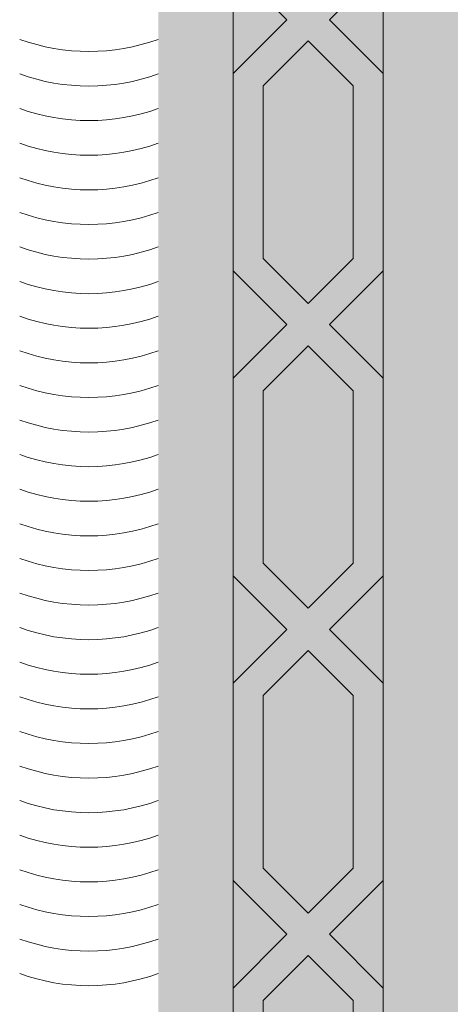
# Model space of a CAD drawing. Units: inches. Extents: x 844 to 2234, y 346 to 1084.
# Tile 27 of 93: x 1249.183 to 1252.862, y 687.38 to 695.763. Entities that reach past the tile are written whole.
import ezdxf

# ---------------------------------------------------------------- set-up
doc = ezdxf.new("R2010")
doc.units = ezdxf.units.IN
doc.header["$MEASUREMENT"] = 0
doc.layers.add('furniture', color=8, linetype='Continuous', lineweight=18)
doc.layers.add('RA-AP-01$0$INT', color=35, linetype='Continuous', lineweight=5)
doc.layers.add('RA-AP-01$0$FURN', color=3, linetype='Continuous')

# ---------------------------------------------------------------- blocks, each defined once
blk = doc.blocks.new('A$C18D01794')
at = {"layer": 'RA-AP-01$0$INT'}
h = blk.add_hatch(color=256, dxfattribs=at)
h.paths.add_polyline_path([(4.35521, -6.15671), (4.35521, -8.05671), (5.45521, -8.05671), (5.45521, -6.15671)])
h.paths.add_polyline_path([(4.40521, -8.00671), (4.40521, -6.20671), (5.40521, -6.20671), (5.40521, -8.00671)], flags=16)
h = blk.add_hatch(color=256, dxfattribs=at)
h.paths.add_polyline_path([(4.46935, -7.07085), (4.50521, -7.035), (4.50521, -7.10671)])
h.paths.add_polyline_path([(4.45521, -7.085), (4.47692, -7.10671), (4.43349, -7.10671)])
h.paths.add_polyline_path([(4.40521, -7.035), (4.44106, -7.07085), (4.40521, -7.10671)])
h.paths.add_polyline_path([(4.42521, -6.91146), (4.45521, -6.88146), (4.48521, -6.91146), (4.48521, -7.02671), (4.45521, -7.05671), (4.42521, -7.02671)])
h.paths.add_polyline_path([(4.50521, -6.83146), (4.50521, -6.90318), (4.46935, -6.86732)])
h.paths.add_polyline_path([(4.42521, -6.70793), (4.45521, -6.67793), (4.48521, -6.70793), (4.48521, -6.82318), (4.45521, -6.85318), (4.42521, -6.82318)])
h.paths.add_polyline_path([(4.42521, -6.50439), (4.45521, -6.47439), (4.48521, -6.50439), (4.48521, -6.61964), (4.45521, -6.64964), (4.42521, -6.61964)])
h.paths.add_polyline_path([(4.46935, -6.66378), (4.50521, -6.62793), (4.50521, -6.69964)])
h.paths.add_polyline_path([(4.40521, -6.62793), (4.44106, -6.66378), (4.40521, -6.69964)])
h.paths.add_polyline_path([(4.40521, -6.42439), (4.44106, -6.46025), (4.40521, -6.49611)])
h.paths.add_polyline_path([(4.46935, -6.46025), (4.50521, -6.42439), (4.50521, -6.49611)])
h.paths.add_polyline_path([(4.42521, -6.30085), (4.45521, -6.27085), (4.48521, -6.30085), (4.48521, -6.41611), (4.45521, -6.44611), (4.42521, -6.41611)])
h.paths.add_polyline_path([(4.42521, -6.22671), (4.47106, -6.22671), (4.42521, -6.27257)])
h.paths.add_polyline_path([(4.49935, -6.22671), (4.63606, -6.22671), (4.66606, -6.25671), (4.63606, -6.28671), (4.49935, -6.28671), (4.46935, -6.25671)])
h.paths.add_polyline_path([(4.68021, -6.27085), (4.71606, -6.30671), (4.64435, -6.30671)])
h.paths.add_polyline_path([(4.64435, -6.20671), (4.71606, -6.20671), (4.68021, -6.24257)])
h.paths.add_polyline_path([(4.72435, -6.22671), (4.86106, -6.22671), (4.89106, -6.25671), (4.86106, -6.28671), (4.72435, -6.28671), (4.69435, -6.25671)])
h.paths.add_polyline_path([(4.90521, -6.27085), (4.94106, -6.30671), (4.86935, -6.30671)])
h.paths.add_polyline_path([(4.86935, -6.20671), (4.94106, -6.20671), (4.90521, -6.24257)])
h.paths.add_polyline_path([(4.94935, -6.22671), (5.08606, -6.22671), (5.11606, -6.25671), (5.08606, -6.28671), (4.94935, -6.28671), (4.91935, -6.25671)])
h.paths.add_polyline_path([(5.13021, -6.27085), (5.16606, -6.30671), (5.09435, -6.30671)])
h.paths.add_polyline_path([(5.09435, -6.20671), (5.16606, -6.20671), (5.13021, -6.24257)])
h.paths.add_polyline_path([(5.17435, -6.22671), (5.31106, -6.22671), (5.34106, -6.25671), (5.31106, -6.28671), (5.17435, -6.28671), (5.14435, -6.25671)])
h.paths.add_polyline_path([(5.32521, -6.30085), (5.35521, -6.27085), (5.38521, -6.30085), (5.38521, -6.41611), (5.35521, -6.44611), (5.32521, -6.41611)])
h.paths.add_polyline_path([(5.33935, -6.22671), (5.38521, -6.22671), (5.38521, -6.27257)])
h.paths.add_polyline_path([(5.32521, -6.50439), (5.35521, -6.47439), (5.38521, -6.50439), (5.38521, -6.61964), (5.35521, -6.64964), (5.32521, -6.61964)])
h.paths.add_polyline_path([(5.30521, -6.42439), (5.34106, -6.46025), (5.30521, -6.49611)])
h.paths.add_polyline_path([(5.36935, -6.46025), (5.40521, -6.42439), (5.40521, -6.49611)])
h.paths.add_polyline_path([(5.40521, -6.62793), (5.40521, -6.69964), (5.36935, -6.66378)])
h.paths.add_polyline_path([(5.30521, -6.62793), (5.34106, -6.66378), (5.30521, -6.69964)])
h.paths.add_polyline_path([(5.32521, -6.70793), (5.35521, -6.67793), (5.38521, -6.70793), (5.38521, -6.82318), (5.35521, -6.85318), (5.32521, -6.82318)])
h.paths.add_polyline_path([(5.30521, -6.83146), (5.34106, -6.86732), (5.30521, -6.90318)])
h.paths.add_polyline_path([(5.32521, -6.91146), (5.35521, -6.88146), (5.38521, -6.91146), (5.38521, -7.02671), (5.35521, -7.05671), (5.32521, -7.02671)])
h.paths.add_polyline_path([(5.40458, -6.83209, 0.001218), (5.40521, -6.83231), (5.40521, -6.90318), (5.36935, -6.86732)])
h.paths.add_polyline_path([(5.36935, -7.07085), (5.40521, -7.035), (5.40521, -7.10671)])
h.paths.add_polyline_path([(5.35521, -7.085), (5.37692, -7.10671), (5.33349, -7.10671)])
h.paths.add_polyline_path([(5.30521, -7.035), (5.34106, -7.07085), (5.30521, -7.10671)])
h = blk.add_hatch(color=256, dxfattribs=at)
h.paths.add_polyline_path([(4.50521, -6.62793), (4.46935, -6.66378), (4.50521, -6.69964), (4.50521, -6.83146), (4.46935, -6.86732), (4.50521, -6.90318), (4.50521, -7.035), (4.46935, -7.07085), (4.50521, -7.10671), (4.47692, -7.10671), (4.45521, -7.085), (4.43349, -7.10671), (4.40521, -7.10671), (4.44106, -7.07085), (4.40521, -7.035), (4.40521, -6.90318), (4.44106, -6.86732), (4.40521, -6.83146), (4.40521, -6.69964), (4.44106, -6.66378), (4.40521, -6.62793), (4.40521, -6.49611), (4.44106, -6.46025), (4.40521, -6.42439), (4.40521, -6.20671), (4.64435, -6.20671), (4.68021, -6.24257), (4.71606, -6.20671), (4.86935, -6.20671), (4.90521, -6.24257), (4.94106, -6.20671), (5.09435, -6.20671), (5.13021, -6.24257), (5.16606, -6.20671), (5.40521, -6.20671), (5.40521, -6.42439), (5.36935, -6.46025), (5.40521, -6.49611), (5.40521, -6.62793), (5.36935, -6.66378), (5.40521, -6.69964), (5.40521, -6.83146), (5.36935, -6.86732), (5.40521, -6.90318), (5.40521, -7.035), (5.36935, -7.07085), (5.40521, -7.10671), (5.37692, -7.10671), (5.35521, -7.085), (5.33349, -7.10671), (5.30521, -7.10671), (5.34106, -7.07085), (5.30521, -7.035), (5.30521, -6.90318), (5.34106, -6.86732), (5.30521, -6.83146), (5.30521, -6.69964), (5.34106, -6.66378), (5.30521, -6.62793), (5.30521, -6.49611), (5.34106, -6.46025), (5.30521, -6.42439), (5.30521, -6.30671), (5.16606, -6.30671), (5.13021, -6.27085), (5.09435, -6.30671), (4.94106, -6.30671), (4.90521, -6.27085), (4.86935, -6.30671), (4.71606, -6.30671), (4.68021, -6.27085), (4.64435, -6.30671), (4.50521, -6.30671), (4.50521, -6.42439), (4.46935, -6.46025), (4.50521, -6.49611)])
h.paths.add_polyline_path([(4.48521, -6.50439), (4.45521, -6.47439), (4.42521, -6.50439), (4.42521, -6.61964), (4.45521, -6.64964), (4.48521, -6.61964)], flags=16)
h.paths.add_polyline_path([(4.45521, -6.44611), (4.48521, -6.41611), (4.48521, -6.30085), (4.45521, -6.27085), (4.42521, -6.30085), (4.42521, -6.41611)], flags=16)
h.paths.add_polyline_path([(4.45521, -6.67793), (4.42521, -6.70793), (4.42521, -6.82318), (4.45521, -6.85318), (4.48521, -6.82318), (4.48521, -6.70793)], flags=16)
h.paths.add_polyline_path([(4.49935, -6.28671), (4.63606, -6.28671), (4.66606, -6.25671), (4.63606, -6.22671), (4.49935, -6.22671), (4.46935, -6.25671)], flags=16)
h.paths.add_polyline_path([(4.42521, -6.27257), (4.47106, -6.22671), (4.42521, -6.22671)], flags=16)
h.paths.add_polyline_path([(4.45521, -6.88146), (4.42521, -6.91146), (4.42521, -7.02671), (4.45521, -7.05671), (4.48521, -7.02671), (4.48521, -6.91146)], flags=16)
h.paths.add_polyline_path([(4.72435, -6.28671), (4.86106, -6.28671), (4.89106, -6.25671), (4.86106, -6.22671), (4.72435, -6.22671), (4.69435, -6.25671)], flags=16)
h.paths.add_polyline_path([(4.91935, -6.25671), (4.94935, -6.28671), (5.08606, -6.28671), (5.11606, -6.25671), (5.08606, -6.22671), (4.94935, -6.22671)], flags=16)
h.paths.add_polyline_path([(5.14435, -6.25671), (5.17435, -6.28671), (5.31106, -6.28671), (5.34106, -6.25671), (5.31106, -6.22671), (5.17435, -6.22671)], flags=16)
h.paths.add_polyline_path([(5.32521, -6.61964), (5.35521, -6.64964), (5.38521, -6.61964), (5.38521, -6.50439), (5.35521, -6.47439), (5.32521, -6.50439)], flags=16)
h.paths.add_polyline_path([(5.32521, -6.41611), (5.35521, -6.44611), (5.38521, -6.41611), (5.38521, -6.30085), (5.35521, -6.27085), (5.32521, -6.30085)], flags=16)
h.paths.add_polyline_path([(5.32521, -6.70793), (5.32521, -6.82318), (5.35521, -6.85318), (5.38521, -6.82318), (5.38521, -6.70793), (5.35521, -6.67793)], flags=16)
h.paths.add_polyline_path([(5.32521, -6.91146), (5.32521, -7.02671), (5.35521, -7.05671), (5.38521, -7.02671), (5.38521, -6.91146), (5.35521, -6.88146)], flags=16)
h.paths.add_polyline_path([(5.33935, -6.22671), (5.38521, -6.27257), (5.38521, -6.22671)], flags=16)
blk.add_hatch(color=256, dxfattribs=at).paths.add_polyline_path([(4.50521, -6.30671), (5.30521, -6.30671), (5.30521, -7.10671), (5.25521, -7.10671), (5.25521, -6.35671), (4.55521, -6.35671), (4.55521, -7.10671), (4.50521, -7.10671)])
for p, q in [((5.32521, -6.30085), (5.32521, -6.41611)), ((5.38521, -6.41611), (5.38521, -6.30085)), ((5.35521, -6.44611), (5.32521, -6.41611)), ((5.35521, -6.44611), (5.38521, -6.41611)), ((5.34106, -6.46025), (5.30521, -6.42439)), ((5.36935, -6.46025), (5.40521, -6.42439)), ((5.30521, -6.49611), (5.34106, -6.46025)), ((5.40521, -6.49611), (5.36935, -6.46025)), ((5.32521, -6.50439), (5.35521, -6.47439)), ((5.38521, -6.50439), (5.35521, -6.47439)), ((5.32521, -6.61964), (5.32521, -6.50439)), ((5.38521, -6.61964), (5.38521, -6.50439)), ((5.32521, -6.61964), (5.35521, -6.64964)), ((5.38521, -6.61964), (5.35521, -6.64964)), ((5.30521, -6.62793), (5.34106, -6.66378)), ((5.40521, -6.62793), (5.36935, -6.66378)), ((5.30521, -6.69964), (5.34106, -6.66378)), ((5.40521, -6.69964), (5.36935, -6.66378)), ((5.32521, -6.70793), (5.35521, -6.67793)), ((5.38521, -6.70793), (5.35521, -6.67793)), ((5.32521, -6.82318), (5.32521, -6.70793)), ((5.38521, -6.82318), (5.38521, -6.70793)), ((5.32521, -6.82318), (5.35521, -6.85318)), ((5.38521, -6.82318), (5.35521, -6.85318)), ((5.30521, -6.83146), (5.34106, -6.86732)), ((5.40521, -6.83146), (5.36935, -6.86732)), ((5.30521, -6.90318), (5.34106, -6.86732)), ((5.40521, -6.90318), (5.36935, -6.86732)), ((5.32521, -6.91146), (5.35521, -6.88146)), ((5.38521, -6.91146), (5.35521, -6.88146)), ((5.32521, -6.91146), (5.32521, -7.02671)), ((5.38521, -6.91146), (5.38521, -7.02671)), ((5.32521, -7.02671), (5.35521, -7.05671)), ((5.38521, -7.02671), (5.35521, -7.05671)), ((5.30521, -7.035), (5.34106, -7.07085)), ((5.40521, -7.035), (5.36935, -7.07085)), ((5.34106, -7.07085), (5.30521, -7.10671)), ((5.36935, -7.07085), (5.40521, -7.10671))]:
    blk.add_line(p, q, dxfattribs=at)
for points in [[(5.40521, -7.10671), (5.40521, -6.20671)], [(5.30521, -7.10671), (5.30521, -6.30671), (4.50521, -6.30671), (4.50521, -7.10671)]]:
    blk.add_lwpolyline(points, dxfattribs=at)
for centre in [(5.50141, -6.56236), (5.50141, -6.58546), (5.50141, -6.60856), (5.50141, -6.63166), (5.50141, -6.65476), (5.50141, -6.67786), (5.50141, -6.70096), (5.50141, -6.72406), (5.50141, -6.74716), (5.50141, -6.77026), (5.50141, -6.79336), (5.50141, -6.79336), (5.50141, -6.81646), (5.50141, -6.83956), (5.50141, -6.86266), (5.50141, -6.88576), (5.50141, -6.90886), (5.50141, -6.93196), (5.50141, -6.95506), (5.50141, -6.97816), (5.50141, -7.00126), (5.50141, -7.02436), (5.50141, -7.04746), (5.50141, -7.07056), (5.50141, -7.09366), (5.50141, -7.11676), (5.50141, -7.13986), (5.50141, -7.16296), (5.50141, -7.18606)]:
    blk.add_arc(centre, 0.13641, 70.20384, 109.79616, dxfattribs=at)
blk = doc.blocks.new('A$C5D2F253E')
at = {"layer": 'RA-AP-01$0$FURN', "xscale": -0.7999999999883585, "yscale": 0.7999999999883585, "zscale": 0.8, "rotation": 90}
blk.add_blockref('A$C18D01794', (-5.68776, 4.75792), dxfattribs=at)

msp = doc.modelspace()

# ---------------------------------------------------------------- block references
at = {"layer": 'furniture', "xscale": -15.94108302203742, "yscale": 15.94108302203742, "zscale": 15.94108302203742, "rotation": 270}
msp.add_blockref('A$C5D2F253E', (1244.0841, 696.2585), dxfattribs=at)

doc.saveas('drawing.dxf')
